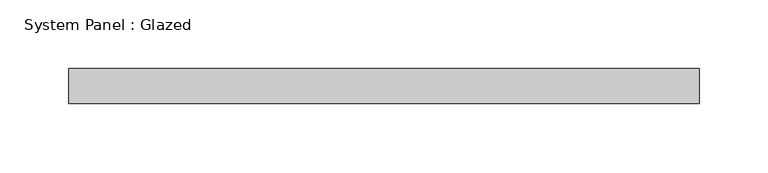
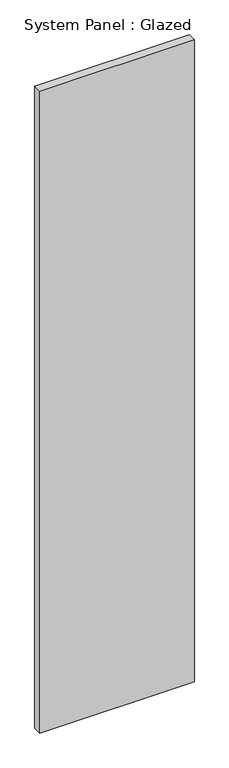
"""IFC4 building model written with IfcOpenShell, lengths in millimetres: plate geometry, System Panel : Glazed."""

from ifc_helpers import new_model, si_unit, origin, origin_with_axes, place, context, project, spatial, polyline, outline, extrude, source, transform, mapped, element, save


def system_panel_glazed_a1cd5516(model_context):
    return source(origin(), model_context, "Body", "SweptSolid", [
        extrude(outline(polyline([(228.6, -44.45), (-228.6, -44.45), (-228.6, -19.05), (228.6, -19.05), (228.6, -44.45)])), origin_with_axes(), (0.0, 0.0, 1.0), 2006.6),
    ])


if __name__ == "__main__":
    model = new_model("IFC4")
    model_context = context("Model", 3, world=origin())
    ifc_project = project(units=[si_unit("LENGTHUNIT", "METRE", prefix="MILLI")], contexts=[model_context])
    site = spatial("IfcSite", under=ifc_project)
    building = spatial("IfcBuilding", under=site)
    placement = place(None, origin())
    system_panel_glazed_shape = system_panel_glazed_a1cd5516(model_context)
    element("IfcPlate", 1, ObjectType="System Panel : Glazed", at=placement, inside=building, context=model_context, shape_type="MappedRepresentation", body=[
        mapped(system_panel_glazed_shape, transform((0.0, 0.0, 0.0), x_axis=(1.0, 0.0, 0.0), y_axis=(0.0, 1.0, 0.0), z_axis=(0.0, 0.0, 1.0))),
    ])
    save(model, "model.ifc")

# Revit data of these elements
# Type "System Panel : Glazed"
#   Construction Type Id = "GSP4R"
#   Analytic Construction = "1/8 in Pilkington single glazing"
#   Visual Light Transmittance = 0.9
#   Solar Heat Gain Coefficient = 0.86
#   Heat Transfer Coefficient (U) = 1.18115 BTU/(h·ft²·°F)
#   Define Thermal Properties by = 1
# Element 1 (IfcPlate, "System Panel : Glazed")
#   Materials on its faces: "Glass"
# Materials
#   "Glass": class "Glass", colour RGB 0 128 192, transparency 0.75, Description = "Soda Lime Glass", Cost = 0
